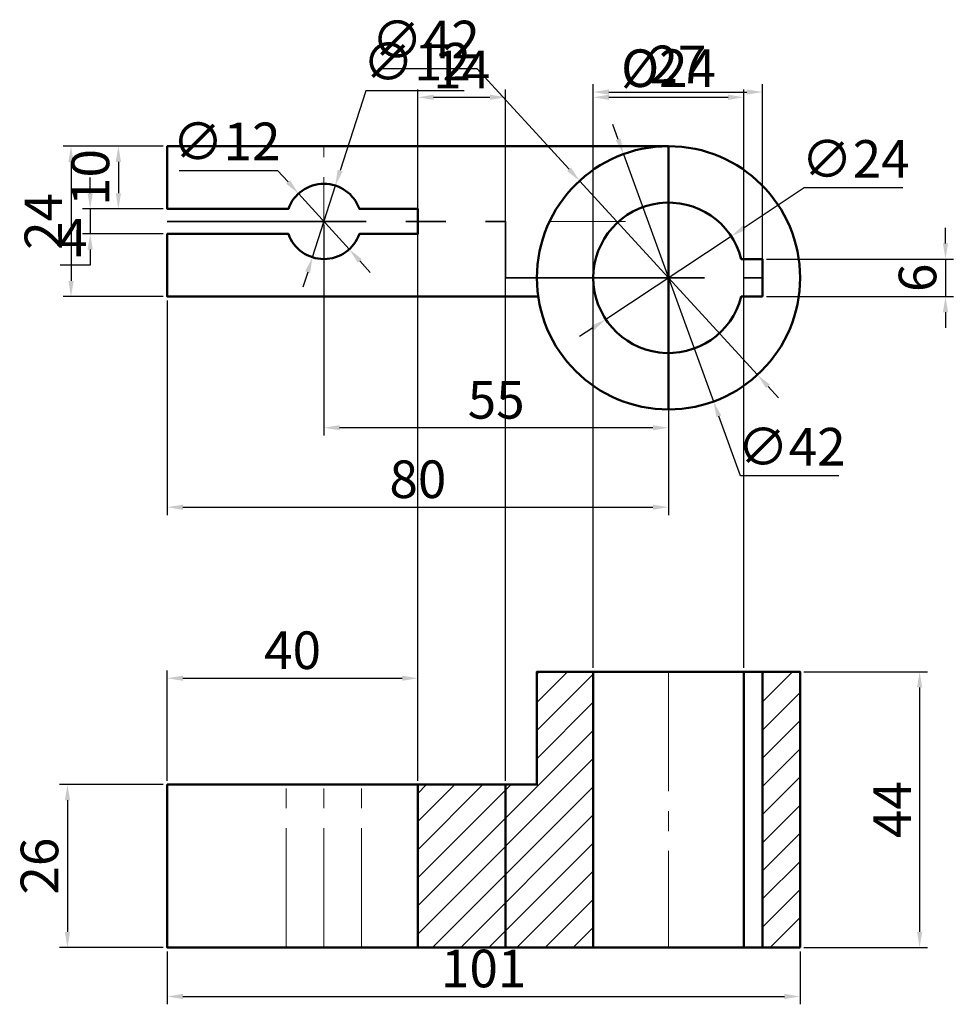
# Model space of a CAD drawing. Units: millimetres. Extents: x 158 to 307, y 11 to 168.
import ezdxf

# ---------------------------------------------------------------- set-up
doc = ezdxf.new("R2010")
doc.units = ezdxf.units.MM
doc.linetypes.add('CENTER2', pattern=[28.575, 19.05, -3.175, 3.175, -3.175])
doc.linetypes.add('PHANTOM', pattern=[63.5, 31.75, -6.35, 6.35, -6.35, 6.35, -6.35])
for name, color, linetype, lineweight in [('M-CNTR', 4, 'CENTER2', 18), ('M-DIMS', 2, 'Continuous', 25), ('M-HATC', 8, 'Continuous', 18), ('M-OUTL', 7, 'Continuous', 50), ('M-SECT', 1, 'PHANTOM', 35)]:
    doc.layers.add(name, color=color, linetype=linetype, lineweight=lineweight)
doc.styles.get("Standard").update_dxf_attribs({"font": 'arial.ttf'})
doc.dimstyles.new('ISO-25', dxfattribs={"dimtxt": 6, "dimasz": 2.5, "dimexe": 1.25, "dimexo": 0.625, "dimtad": 1, "dimtoh": 1, "dimdec": 0, "dimtxsty": 'Standard', "dimcen": 2.5, "dimadec": 0, "dimazin": 0, "dimtfac": 1, "dimtdec": 0, "dimtmove": 0, "dimatfit": 3, "dimfxl": 1, "dimarcsym": 0})

# ---------------------------------------------------------------- blocks, each defined once
blk = doc.blocks.new('*D1')
at = {"layer": 'Defpoints', "color": 0, "transparency": 16777216}
for p in [(221.54, 62.82), (181.54, 45.85), (221.54, 45.85)]:
    blk.add_point(p, dxfattribs=at)
at = {"layer": 'M-DIMS', "color": 0, "lineweight": -2, "transparency": 16777216}
for p, q in [((181.54, 46.48), (181.54, 64.07)), ((221.54, 46.48), (221.54, 64.07)), ((184.04, 62.82), (219.04, 62.82))]:
    blk.add_line(p, q, dxfattribs=at)
at = {"layer": 'M-DIMS', "color": 0, "transparency": 16777216}
for points in [[(184.04, 63.24), (184.04, 62.41), (181.54, 62.82)], [(219.04, 63.24), (219.04, 62.41), (221.54, 62.82)]]:
    blk.add_solid(points, dxfattribs=at)
at = {"layer": 'M-DIMS', "color": 0, "transparency": 16777216, "insert": (201.54, 66.51), "char_height": 6, "attachment_point": 5}
blk.add_mtext('40', dxfattribs=at)
blk = doc.blocks.new('*D2')
at = {"layer": 'Defpoints', "color": 0, "transparency": 16777216}
for p in [(282.54, 63.85), (282.54, 19.85), (301.62, 19.85)]:
    blk.add_point(p, dxfattribs=at)
at = {"layer": 'M-DIMS', "color": 0, "lineweight": -2, "transparency": 16777216}
for p, q in [((283.16, 63.85), (302.87, 63.85)), ((301.62, 61.35), (301.62, 22.35)), ((283.16, 19.85), (302.87, 19.85))]:
    blk.add_line(p, q, dxfattribs=at)
at = {"layer": 'M-DIMS', "color": 0, "transparency": 16777216}
for points in [[(301.2, 61.35), (302.04, 61.35), (301.62, 63.85)], [(301.2, 22.35), (302.04, 22.35), (301.62, 19.85)]]:
    blk.add_solid(points, dxfattribs=at)
at = {"layer": 'M-DIMS', "color": 0, "transparency": 16777216, "insert": (298, 41.85), "char_height": 6, "attachment_point": 5, "rotation": 90}
blk.add_mtext('44', dxfattribs=at)
blk = doc.blocks.new('*D3')
at = {"layer": 'Defpoints', "color": 0, "transparency": 16777216}
for p in [(181.54, 45.85), (165.61, 19.85), (181.54, 19.85)]:
    blk.add_point(p, dxfattribs=at)
at = {"layer": 'M-DIMS', "color": 0, "lineweight": -2, "transparency": 16777216}
for p, q in [((180.91, 45.85), (164.36, 45.85)), ((165.61, 43.35), (165.61, 22.35)), ((180.91, 19.85), (164.36, 19.85))]:
    blk.add_line(p, q, dxfattribs=at)
at = {"layer": 'M-DIMS', "color": 0, "transparency": 16777216}
for points in [[(165.19, 43.35), (166.03, 43.35), (165.61, 45.85)], [(165.19, 22.35), (166.03, 22.35), (165.61, 19.85)]]:
    blk.add_solid(points, dxfattribs=at)
at = {"layer": 'M-DIMS', "color": 0, "transparency": 16777216, "insert": (161.92, 32.85), "char_height": 6, "attachment_point": 5, "rotation": 90}
blk.add_mtext('26', dxfattribs=at)
blk = doc.blocks.new('*D4')
at = {"layer": 'Defpoints', "color": 0, "transparency": 16777216}
for p in [(181.54, 123.7), (261.54, 123.7), (261.54, 90.11)]:
    blk.add_point(p, dxfattribs=at)
at = {"layer": 'M-DIMS', "color": 0, "lineweight": -2, "transparency": 16777216}
for p, q in [((181.54, 123.08), (181.54, 88.86)), ((261.54, 123.08), (261.54, 88.86)), ((184.04, 90.11), (259.04, 90.11))]:
    blk.add_line(p, q, dxfattribs=at)
at = {"layer": 'M-DIMS', "color": 0, "transparency": 16777216}
for points in [[(184.04, 90.52), (184.04, 89.69), (181.54, 90.11)], [(259.04, 90.52), (259.04, 89.69), (261.54, 90.11)]]:
    blk.add_solid(points, dxfattribs=at)
at = {"layer": 'M-DIMS', "color": 0, "transparency": 16777216, "insert": (221.54, 93.79), "char_height": 6, "attachment_point": 5}
blk.add_mtext('80', dxfattribs=at)
blk = doc.blocks.new('*D5')
at = {"layer": 'Defpoints', "color": 0, "transparency": 16777216}
for p in [(181.54, 147.7), (166.18, 123.7), (181.54, 123.7)]:
    blk.add_point(p, dxfattribs=at)
at = {"layer": 'M-DIMS', "color": 0, "lineweight": -2, "transparency": 16777216}
for p, q in [((180.91, 147.7), (164.93, 147.7)), ((166.18, 145.2), (166.18, 126.2)), ((180.91, 123.7), (164.93, 123.7))]:
    blk.add_line(p, q, dxfattribs=at)
at = {"layer": 'M-DIMS', "color": 0, "transparency": 16777216}
for points in [[(165.76, 145.2), (166.6, 145.2), (166.18, 147.7)], [(165.76, 126.2), (166.6, 126.2), (166.18, 123.7)]]:
    blk.add_solid(points, dxfattribs=at)
at = {"layer": 'M-DIMS', "color": 0, "transparency": 16777216, "insert": (162.54, 135.7), "char_height": 6, "attachment_point": 5, "rotation": 90}
blk.add_mtext('24', dxfattribs=at)
blk = doc.blocks.new('*D6')
at = {"layer": 'Defpoints', "color": 0, "transparency": 16777216}
for p in [(181.54, 137.7), (169.24, 133.7), (181.54, 133.7)]:
    blk.add_point(p, dxfattribs=at)
at = {"layer": 'M-DIMS', "color": 0, "lineweight": -2, "transparency": 16777216}
for p, q in [((169.24, 140.2), (169.24, 142.7)), ((180.91, 137.7), (167.99, 137.7)), ((169.24, 137.7), (169.24, 133.7)), ((180.91, 133.7), (167.99, 133.7)), ((169.24, 131.2), (169.24, 128.7)), ((169.24, 128.7), (164.47, 128.7))]:
    blk.add_line(p, q, dxfattribs=at)
at = {"layer": 'M-DIMS', "color": 0, "transparency": 16777216}
for points in [[(168.82, 140.2), (169.66, 140.2), (169.24, 137.7)], [(168.82, 131.2), (169.66, 131.2), (169.24, 133.7)]]:
    blk.add_solid(points, dxfattribs=at)
at = {"layer": 'M-DIMS', "color": 0, "transparency": 16777216, "insert": (166.54, 132.33), "char_height": 6, "attachment_point": 5}
blk.add_mtext('4', dxfattribs=at)
blk = doc.blocks.new('*D7')
at = {"layer": 'Defpoints', "color": 0, "transparency": 16777216}
for p in [(276.54, 156.34), (249.54, 126.7), (276.54, 126.7)]:
    blk.add_point(p, dxfattribs=at)
at = {"layer": 'M-DIMS', "color": 0, "lineweight": -2, "transparency": 16777216}
for p, q in [((249.54, 127.33), (249.54, 157.59)), ((276.54, 127.33), (276.54, 157.59)), ((252.04, 156.34), (274.04, 156.34))]:
    blk.add_line(p, q, dxfattribs=at)
at = {"layer": 'M-DIMS', "color": 0, "transparency": 16777216}
for points in [[(252.04, 156.75), (252.04, 155.92), (249.54, 156.34)], [(274.04, 156.75), (274.04, 155.92), (276.54, 156.34)]]:
    blk.add_solid(points, dxfattribs=at)
at = {"layer": 'M-DIMS', "color": 0, "transparency": 16777216, "insert": (263.04, 159.97), "char_height": 6, "attachment_point": 5}
blk.add_mtext('27', dxfattribs=at)
blk = doc.blocks.new('*D8')
at = {"layer": 'Defpoints', "color": 0, "transparency": 16777216}
for p in [(276.54, 129.7), (276.54, 123.7), (305.75, 123.7)]:
    blk.add_point(p, dxfattribs=at)
at = {"layer": 'M-DIMS', "color": 0, "lineweight": -2, "transparency": 16777216}
for p, q in [((305.75, 132.2), (305.75, 134.7)), ((277.16, 129.7), (307, 129.7)), ((305.75, 129.7), (305.75, 123.7)), ((277.16, 123.7), (307, 123.7)), ((305.75, 121.2), (305.75, 118.7))]:
    blk.add_line(p, q, dxfattribs=at)
at = {"layer": 'M-DIMS', "color": 0, "transparency": 16777216}
for points in [[(305.33, 132.2), (306.16, 132.2), (305.75, 129.7)], [(305.33, 121.2), (306.16, 121.2), (305.75, 123.7)]]:
    blk.add_solid(points, dxfattribs=at)
at = {"layer": 'M-DIMS', "color": 0, "transparency": 16777216, "insert": (302.06, 126.7), "char_height": 6, "attachment_point": 5, "rotation": 90}
blk.add_mtext('6', dxfattribs=at)
blk = doc.blocks.new('*D9')
at = {"layer": 'Defpoints', "color": 0, "transparency": 16777216}
for p in [(206.54, 135.7), (261.54, 126.7), (206.54, 102.78)]:
    blk.add_point(p, dxfattribs=at)
at = {"layer": 'M-DIMS', "color": 0, "lineweight": -2, "transparency": 16777216}
for p, q in [((206.54, 135.08), (206.54, 101.53)), ((261.54, 126.08), (261.54, 101.53)), ((259.04, 102.78), (209.04, 102.78))]:
    blk.add_line(p, q, dxfattribs=at)
at = {"layer": 'M-DIMS', "color": 0, "transparency": 16777216}
for points in [[(209.04, 103.2), (209.04, 102.37), (206.54, 102.78)], [(259.04, 103.2), (259.04, 102.37), (261.54, 102.78)]]:
    blk.add_solid(points, dxfattribs=at)
at = {"layer": 'M-DIMS', "color": 0, "transparency": 16777216, "insert": (234.04, 106.46), "char_height": 6, "attachment_point": 5}
blk.add_mtext('55', dxfattribs=at)
blk = doc.blocks.new('*D10')
at = {"layer": 'Defpoints', "color": 0, "transparency": 16777216}
for p in [(208.37, 141.42), (204.71, 129.99)]:
    blk.add_point(p, dxfattribs=at)
at = {"layer": 'M-DIMS', "color": 0, "lineweight": -2, "transparency": 16777216}
for p, q in [((213.21, 156.55), (209.13, 143.8)), ((228.9, 156.55), (213.21, 156.55)), ((204.71, 129.99), (208.37, 141.42)), ((203.95, 127.61), (203.19, 125.22))]:
    blk.add_line(p, q, dxfattribs=at)
at = {"layer": 'M-DIMS', "color": 0, "transparency": 16777216}
for points in [[(208.73, 143.92), (209.53, 143.67), (208.37, 141.42)], [(203.55, 127.73), (204.35, 127.48), (204.71, 129.99)]]:
    blk.add_solid(points, dxfattribs=at)
at = {"layer": 'M-DIMS', "color": 0, "transparency": 16777216, "insert": (221.37, 160.41), "char_height": 6, "attachment_point": 5}
blk.add_mtext('∅12', dxfattribs=at)
blk = doc.blocks.new('*D11')
at = {"layer": 'Defpoints', "color": 0, "transparency": 16777216}
for p in [(247.35, 142.18), (275.73, 111.22)]:
    blk.add_point(p, dxfattribs=at)
at = {"layer": 'M-DIMS', "color": 0, "lineweight": -2, "transparency": 16777216}
for p, q in [((215.24, 160.09), (230.93, 160.09)), ((230.93, 160.09), (245.66, 144.02)), ((275.73, 111.22), (247.35, 142.18)), ((277.42, 109.38), (279.11, 107.54))]:
    blk.add_line(p, q, dxfattribs=at)
at = {"layer": 'M-DIMS', "color": 0, "transparency": 16777216}
for points in [[(245.97, 144.3), (245.35, 143.74), (247.35, 142.18)], [(277.73, 109.66), (277.11, 109.1), (275.73, 111.22)]]:
    blk.add_solid(points, dxfattribs=at)
at = {"layer": 'M-DIMS', "color": 0, "transparency": 16777216, "insert": (222.78, 163.94), "char_height": 6, "attachment_point": 5}
blk.add_mtext('∅42', dxfattribs=at)
blk = doc.blocks.new('*D12')
at = {"layer": 'Defpoints', "color": 0, "transparency": 16777216}
for p in [(271.55, 133.32), (251.53, 120.08)]:
    blk.add_point(p, dxfattribs=at)
at = {"layer": 'M-DIMS', "color": 0, "lineweight": -2, "transparency": 16777216}
for p, q in [((283.21, 141.03), (273.63, 134.7)), ((298.94, 141.03), (283.21, 141.03)), ((251.53, 120.08), (271.55, 133.32)), ((249.45, 118.7), (247.36, 117.32))]:
    blk.add_line(p, q, dxfattribs=at)
at = {"layer": 'M-DIMS', "color": 0, "transparency": 16777216}
for points in [[(273.4, 135.05), (273.86, 134.35), (271.55, 133.32)], [(249.22, 119.05), (249.68, 118.36), (251.53, 120.08)]]:
    blk.add_solid(points, dxfattribs=at)
at = {"layer": 'M-DIMS', "color": 0, "transparency": 16777216, "insert": (291.39, 144.89), "char_height": 6, "attachment_point": 5}
blk.add_mtext('∅24', dxfattribs=at)
blk = doc.blocks.new('*D13')
at = {"layer": 'Defpoints', "color": 0, "transparency": 16777216}
for p in [(273.54, 155.5), (249.54, 63.85), (273.54, 63.85)]:
    blk.add_point(p, dxfattribs=at)
at = {"layer": 'M-DIMS', "color": 0, "lineweight": -2, "transparency": 16777216}
for p, q in [((249.54, 64.48), (249.54, 156.75)), ((273.54, 64.48), (273.54, 156.75)), ((252.04, 155.5), (271.04, 155.5))]:
    blk.add_line(p, q, dxfattribs=at)
at = {"layer": 'M-DIMS', "color": 0, "transparency": 16777216}
for points in [[(252.04, 155.92), (252.04, 155.08), (249.54, 155.5)], [(271.04, 155.92), (271.04, 155.08), (273.54, 155.5)]]:
    blk.add_solid(points, dxfattribs=at)
at = {"layer": 'M-DIMS', "color": 0, "transparency": 16777216, "insert": (261.54, 159.36), "char_height": 6, "attachment_point": 5}
blk.add_mtext('%%c24', dxfattribs=at)
blk = doc.blocks.new('*D14')
at = {"layer": 'Defpoints', "color": 0, "transparency": 16777216}
for p in [(181.54, 19.85), (282.54, 19.85), (282.54, 12.05)]:
    blk.add_point(p, dxfattribs=at)
at = {"layer": 'M-DIMS', "color": 0, "lineweight": -2, "transparency": 16777216}
for p, q in [((181.54, 19.23), (181.54, 10.8)), ((282.54, 19.23), (282.54, 10.8)), ((184.04, 12.05), (280.04, 12.05))]:
    blk.add_line(p, q, dxfattribs=at)
at = {"layer": 'M-DIMS', "color": 0, "transparency": 16777216}
for points in [[(184.04, 12.47), (184.04, 11.64), (181.54, 12.05)], [(280.04, 12.47), (280.04, 11.64), (282.54, 12.05)]]:
    blk.add_solid(points, dxfattribs=at)
at = {"layer": 'M-DIMS', "color": 0, "transparency": 16777216, "insert": (232.04, 15.74), "char_height": 6, "attachment_point": 5}
blk.add_mtext('101', dxfattribs=at)
blk = doc.blocks.new('*D15')
at = {"layer": 'Defpoints', "color": 0, "transparency": 16777216}
for p in [(235.54, 155.5), (221.54, 45.85), (235.54, 45.85)]:
    blk.add_point(p, dxfattribs=at)
at = {"layer": 'M-DIMS', "color": 0, "lineweight": -2, "transparency": 16777216}
for p, q in [((221.54, 46.48), (221.54, 156.75)), ((235.54, 46.48), (235.54, 156.75)), ((224.04, 155.5), (233.04, 155.5))]:
    blk.add_line(p, q, dxfattribs=at)
at = {"layer": 'M-DIMS', "color": 0, "transparency": 16777216}
for points in [[(224.04, 155.92), (224.04, 155.08), (221.54, 155.5)], [(233.04, 155.92), (233.04, 155.08), (235.54, 155.5)]]:
    blk.add_solid(points, dxfattribs=at)
at = {"layer": 'M-DIMS', "color": 0, "transparency": 16777216, "insert": (228.54, 159.14), "char_height": 6, "attachment_point": 5}
blk.add_mtext('14', dxfattribs=at)
blk = doc.blocks.new('*D16')
at = {"layer": 'Defpoints', "color": 0, "transparency": 16777216}
for p in [(181.54, 147.7), (173.74, 137.7), (181.54, 137.7)]:
    blk.add_point(p, dxfattribs=at)
at = {"layer": 'M-DIMS', "color": 0, "lineweight": -2, "transparency": 16777216}
for p, q in [((180.91, 147.7), (172.49, 147.7)), ((173.74, 145.2), (173.74, 140.2)), ((180.91, 137.7), (172.49, 137.7))]:
    blk.add_line(p, q, dxfattribs=at)
at = {"layer": 'M-DIMS', "color": 0, "transparency": 16777216}
for points in [[(173.32, 145.2), (174.16, 145.2), (173.74, 147.7)], [(173.32, 140.2), (174.16, 140.2), (173.74, 137.7)]]:
    blk.add_solid(points, dxfattribs=at)
at = {"layer": 'M-DIMS', "color": 0, "transparency": 16777216, "insert": (170.05, 142.7), "char_height": 6, "attachment_point": 5, "rotation": 90}
blk.add_mtext('10', dxfattribs=at)
blk = doc.blocks.new('*D17')
at = {"layer": 'Defpoints', "color": 0, "transparency": 16777216}
for p in [(254.36, 146.44), (268.72, 106.97)]:
    blk.add_point(p, dxfattribs=at)
at = {"layer": 'M-DIMS', "color": 0, "lineweight": -2, "transparency": 16777216}
for p, q in [((253.51, 148.79), (252.65, 151.14)), ((254.36, 146.44), (268.72, 106.97)), ((273.02, 95.12), (269.57, 104.62)), ((288.71, 95.12), (273.02, 95.12))]:
    blk.add_line(p, q, dxfattribs=at)
at = {"layer": 'M-DIMS', "color": 0, "transparency": 16777216}
for points in [[(253.9, 148.93), (253.12, 148.64), (254.36, 146.44)], [(269.96, 104.76), (269.18, 104.47), (268.72, 106.97)]]:
    blk.add_solid(points, dxfattribs=at)
at = {"layer": 'M-DIMS', "color": 0, "transparency": 16777216, "insert": (281.18, 98.98), "char_height": 6, "attachment_point": 5}
blk.add_mtext('∅42', dxfattribs=at)
blk = doc.blocks.new('*D18')
at = {"layer": 'Defpoints', "color": 0, "transparency": 16777216}
for p in [(202.5, 140.14), (210.58, 131.26)]:
    blk.add_point(p, dxfattribs=at)
at = {"layer": 'M-DIMS', "color": 0, "lineweight": -2, "transparency": 16777216}
for p, q in [((183.45, 143.84), (199.14, 143.84)), ((199.14, 143.84), (200.82, 141.99)), ((210.58, 131.26), (202.5, 140.14)), ((212.26, 129.41), (213.94, 127.57))]:
    blk.add_line(p, q, dxfattribs=at)
at = {"layer": 'M-DIMS', "color": 0, "transparency": 16777216}
for points in [[(201.13, 142.27), (200.51, 141.71), (202.5, 140.14)], [(212.57, 129.7), (211.95, 129.13), (210.58, 131.26)]]:
    blk.add_solid(points, dxfattribs=at)
at = {"layer": 'M-DIMS', "color": 0, "transparency": 16777216, "insert": (190.98, 147.69), "char_height": 6, "attachment_point": 5}
blk.add_mtext('∅12', dxfattribs=at)

msp = doc.modelspace()

# ---------------------------------------------------------------- hatches: boundary and pattern name
at = {"layer": 'M-HATC'}
h = msp.add_hatch(dxfattribs=at)
h.set_pattern_fill('ANSI31', color=256)
h.set_pattern_definition([(45, (154.639, 0), (-2.245064, 2.245064), [])])
h.paths.add_polyline_path([(249.54, 63.85), (240.54, 63.85), (240.54, 45.85), (235.54, 45.85), (235.54, 19.85), (249.54, 19.85)])
h.paths.add_polyline_path([(235.54, 45.85), (221.54, 45.85), (221.54, 19.85), (235.54, 19.85)])
h.paths.add_polyline_path([(282.54, 63.85), (276.54, 63.85), (276.54, 19.85), (282.54, 19.85)])

# ---------------------------------------------------------------- linework, layer by layer
at = {"layer": 'M-CNTR'}
for p, q in [((206.54, 123.7), (206.54, 147.7)), ((242.57, 135.7), (254.65, 135.7)), ((261.54, 63.85), (261.54, 19.85)), ((200.54, 19.85), (200.54, 45.85)), ((206.54, 19.85), (206.54, 45.85)), ((212.54, 19.85), (212.54, 45.85))]:
    msp.add_line(p, q, dxfattribs=at)
at = {"layer": 'M-OUTL'}
for p, q in [((249.54, 63.85), (249.54, 19.85)), ((273.54, 63.85), (273.54, 19.85)), ((276.54, 63.85), (276.54, 19.85)), ((221.54, 45.85), (221.54, 19.85)), ((235.54, 45.85), (235.54, 19.85))]:
    msp.add_line(p, q, dxfattribs=at)
msp.add_lwpolyline([(261.54, 105.7), (261.54, 147.7), (181.54, 147.7), (181.54, 137.7), (200.88, 137.7, -0.707107), (212.2, 137.7), (221.54, 137.7), (221.54, 133.7), (212.2, 133.7, -0.707107), (200.88, 133.7), (181.54, 133.7), (181.54, 123.7), (240.76, 123.7)], format="xyb", dxfattribs=at)
msp.add_lwpolyline([(276.54, 123.7), (273.16, 123.7, -7.872983), (273.16, 129.7), (276.54, 129.7)], format="xyb", close=True, dxfattribs=at)
msp.add_lwpolyline([(282.54, 19.85), (282.54, 63.85), (240.54, 63.85), (240.54, 45.85), (181.54, 45.85), (181.54, 19.85)], close=True, dxfattribs=at)
msp.add_circle((261.54, 126.7), 21, dxfattribs=at)
at = {"layer": 'M-SECT'}
msp.add_lwpolyline([(181.54, 135.7), (235.54, 135.7), (235.54, 126.7), (276.54, 126.7)], dxfattribs=at)

# ---------------------------------------------------------------- dimensions: what is measured, and where the dimension line sits
at = {"layer": 'M-DIMS'}
for p1, p2, override, picture, middle in [((275.73, 111.22), (247.35, 142.18), {"dimclrd": 0, "dimclre": 0, "dimclrt": 0}, '*D11', (222.78, 160.09)), ((204.71, 129.99), (208.37, 141.42), {"dimclrd": 0, "dimclre": 0, "dimclrt": 0}, '*D10', (221.37, 156.55)), ((210.58, 131.26), (202.5, 140.14), {"dimdec": 0, "dimlfac": 1, "dimrnd": 0, "dimzin": 0, "dimdsep": 46, "dimlunit": 2}, '*D18', (190.98, 143.84)), ((254.36, 146.44), (268.72, 106.97), {"dimdec": 0, "dimlfac": 1, "dimrnd": 0, "dimzin": 0, "dimdsep": 46, "dimlunit": 2}, '*D17', (281.18, 95.12)), ((251.53, 120.08), (271.55, 133.32), {"dimclrd": 0, "dimclre": 0, "dimclrt": 0}, '*D12', (291.39, 141.03))]:
    dim = msp.add_diameter_dim_2p(p1=p1, p2=p2, dimstyle='ISO-25', override=override, dxfattribs=at)
    dim.commit()
    dim.dimension.update_dxf_attribs({"geometry": picture, "text_midpoint": middle, "dimtype": 163})
for base, p1, p2, override, picture, middle in [((276.54, 156.34), (249.54, 126.7), (276.54, 126.7), {"dimclrd": 0, "dimclre": 0, "dimclrt": 0}, '*D7', (263.04, 159.97)), ((235.54, 155.5), (221.54, 45.85), (235.54, 45.85), {"dimdec": 0, "dimlfac": 1, "dimrnd": 0, "dimzin": 0, "dimdsep": 46, "dimlunit": 2}, '*D15', (228.54, 159.14)), ((206.54, 102.78), (261.54, 126.7), (206.54, 135.7), {"dimclrd": 0, "dimclre": 0, "dimclrt": 0}, '*D9', (234.04, 106.46)), ((261.54, 90.11), (181.54, 123.7), (261.54, 123.7), {"dimclrd": 0, "dimclre": 0, "dimclrt": 0}, '*D4', (221.54, 93.79)), ((221.54, 62.82), (181.54, 45.85), (221.54, 45.85), {"dimclrd": 0, "dimclre": 0, "dimclrt": 0}, '*D1', (201.54, 66.51)), ((282.54, 12.05), (181.54, 19.85), (282.54, 19.85), {"dimdec": 0, "dimlfac": 1, "dimrnd": 0, "dimzin": 0, "dimdsep": 46, "dimlunit": 2}, '*D14', (232.04, 15.74))]:
    dim = msp.add_linear_dim(base=base, p1=p1, p2=p2, dimstyle='ISO-25', override=override, dxfattribs=at)
    dim.commit()
    dim.dimension.update_dxf_attribs({"geometry": picture, "text_midpoint": middle})
dim = msp.add_linear_dim(base=(273.54, 155.5), p1=(249.54, 63.85), p2=(273.54, 63.85), text='%%c<>', dimstyle='ISO-25', override={"dimdec": 0, "dimlfac": 1, "dimrnd": 0, "dimzin": 0, "dimdsep": 46, "dimlunit": 2}, dxfattribs=at)
dim.commit()
dim.dimension.update_dxf_attribs({"geometry": '*D13', "text_midpoint": (261.54, 159.36)})
for base, p1, p2, override, picture, middle in [((166.18, 123.7), (181.54, 147.7), (181.54, 123.7), {"dimclrd": 0, "dimclre": 0, "dimclrt": 0}, '*D5', (162.54, 135.7)), ((173.74, 137.7), (181.54, 147.7), (181.54, 137.7), {"dimdec": 0, "dimlfac": 1, "dimrnd": 0, "dimzin": 0, "dimdsep": 46, "dimlunit": 2}, '*D16', (170.05, 142.7)), ((169.24, 133.7), (181.54, 137.7), (181.54, 133.7), {"dimclrd": 0, "dimclre": 0, "dimclrt": 0}, '*D6', (166.54, 132.33)), ((305.75, 123.7), (276.54, 129.7), (276.54, 123.7), {"dimclrd": 0, "dimclre": 0, "dimclrt": 0}, '*D8', (302.06, 126.7)), ((301.62, 19.85), (282.54, 63.85), (282.54, 19.85), {"dimclrd": 0, "dimclre": 0, "dimclrt": 0}, '*D2', (298, 41.85)), ((165.61, 19.85), (181.54, 45.85), (181.54, 19.85), {"dimclrd": 0, "dimclre": 0, "dimclrt": 0}, '*D3', (161.92, 32.85))]:
    dim = msp.add_linear_dim(base=base, p1=p1, p2=p2, angle=90, dimstyle='ISO-25', override=override, dxfattribs=at)
    dim.commit()
    dim.dimension.update_dxf_attribs({"geometry": picture, "text_midpoint": middle})

doc.saveas('drawing.dxf')
